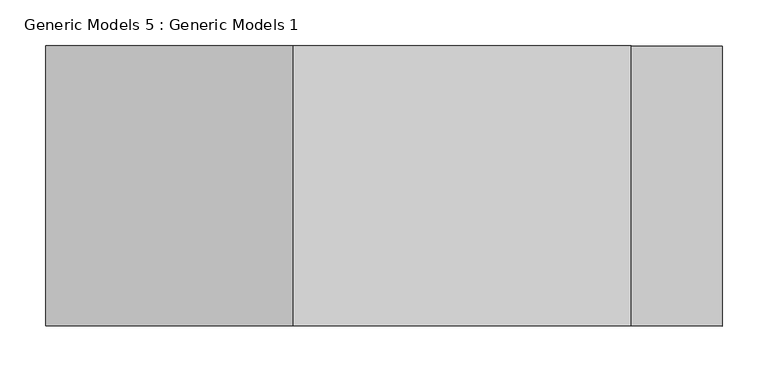
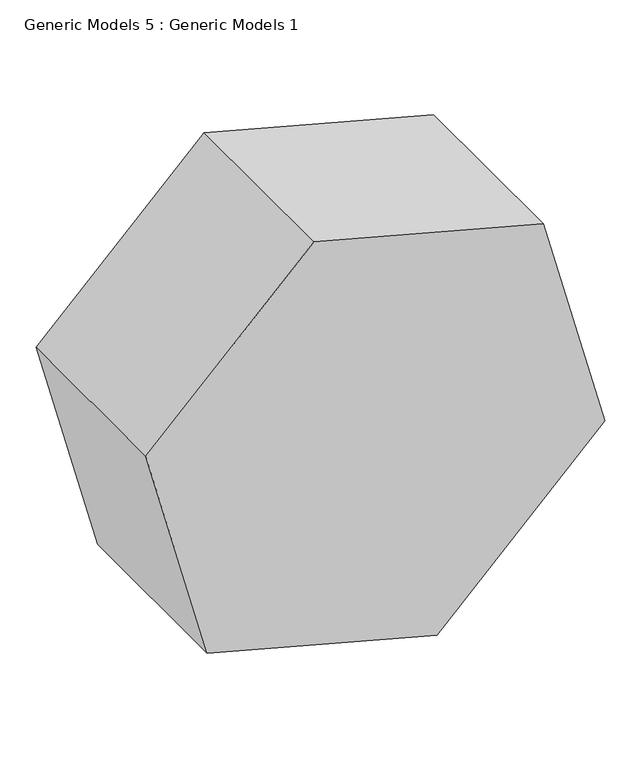
"""IFC4 building model written with IfcOpenShell, lengths in millimetres: proxy geometry, Generic Models 5 : Generic Models 1."""

from ifc_helpers import new_model, si_unit, frame, origin, place, context, project, spatial, polyline, outline, extrude, source, transform, mapped, element, save


def generic_models_5_generic_models_1_6e22be36(model_context):
    return source(origin(), model_context, "Body", "SweptSolid", [
        extrude(outline(polyline([(904.7566299, -6291.8070438), (1003.366686, -6659.8247836), (733.9590024, -6929.2324672), (365.9412626, -6830.622411), (267.3312064, -6462.6046712), (536.73889, -6193.1969876), (904.7566299, -6291.8070438)])), frame((0.0, -9086.6225464, 0.0), z_axis=(0.0, 1.0, 0.0), x_axis=(0.0, 0.0, 1.0)), (0.0, 0.0, 1.0), 304.8),
    ])


if __name__ == "__main__":
    model = new_model("IFC4")
    model_context = context("Model", 3, world=origin())
    ifc_project = project(units=[si_unit("LENGTHUNIT", "METRE", prefix="MILLI")], contexts=[model_context])
    site = spatial("IfcSite", under=ifc_project)
    building = spatial("IfcBuilding", under=site)
    placement = place(None, origin())
    generic_models_5_generic_models_1_shape = generic_models_5_generic_models_1_6e22be36(model_context)
    element("IfcBuildingElementProxy", 1, Name="Generic Models 5 : Generic Models 1", ObjectType="Generic Models 5 : Generic Models 1", at=placement, inside=building, context=model_context, shape_type="MappedRepresentation", body=[
        mapped(generic_models_5_generic_models_1_shape, transform((0.0, 0.0, 0.0), x_axis=(1.0, 0.0, 0.0), y_axis=(0.0, 1.0, 0.0), z_axis=(0.0, 0.0, 1.0))),
    ])
    save(model, "model.ifc")

# Revit data of these elements
# Element 1 (IfcBuildingElementProxy, "Generic Models 5 : Generic Models 1")
#   Materials on its faces: "Carpet (1)"
# Materials
#   "Carpet (1)": class "Carpet", colour RGB 124 80 67, transparency 0, Description = "Interior finish", Cost = 0
